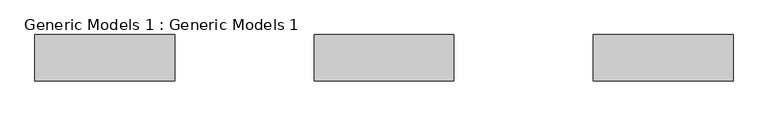
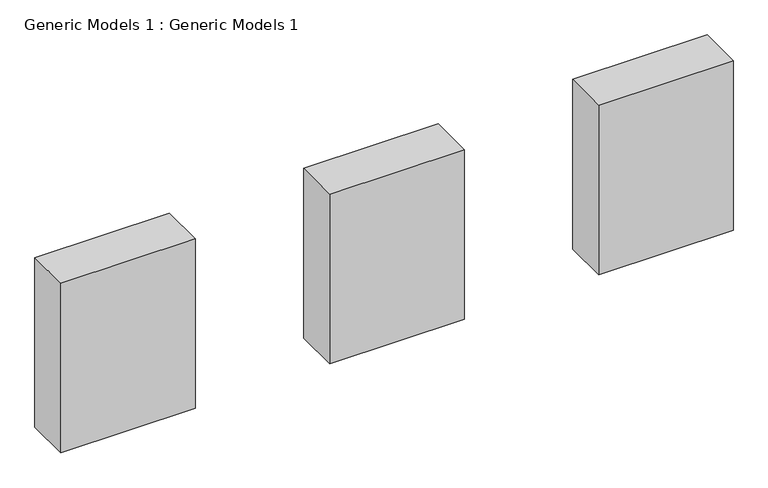
"""IFC4 building model written with IfcOpenShell, lengths in millimetres: proxy geometry, Generic Models 1 : Generic Models 1."""

from ifc_helpers import new_model, si_unit, frame, origin, place, context, project, spatial, polyline, outline, extrude, source, transform, mapped, element, save


def generic_models_1_generic_models_1_0d6a6266(model_context):
    return source(origin(), model_context, "Body", "SweptSolid", [
        extrude(outline(polyline([(-7718.7497054, -8164.8977377), (-8633.1497054, -8164.8977377), (-8633.1497054, -7860.0977377), (-7718.7497054, -7860.0977377), (-7718.7497054, -8164.8977377)])), frame((0.0, 0.0, 129.9820609), z_axis=(0.0, 0.0, 1.0), x_axis=(1.0, 0.0, 0.0)), (0.0, 0.0, 1.0), 1219.2),
        extrude(outline(polyline([(-5889.9497054, -8164.8977377), (-6804.3497054, -8164.8977377), (-6804.3497054, -7860.0977377), (-5889.9497054, -7860.0977377), (-5889.9497054, -8164.8977377)])), frame((0.0, 0.0, 129.9820609), z_axis=(0.0, 0.0, 1.0), x_axis=(1.0, 0.0, 0.0)), (0.0, 0.0, 1.0), 1219.2),
        extrude(outline(polyline([(-4061.1497054, -8164.8977377), (-4975.5497054, -8164.8977377), (-4975.5497054, -7860.0977377), (-4061.1497054, -7860.0977377), (-4061.1497054, -8164.8977377)])), frame((0.0, 0.0, 129.9820609), z_axis=(0.0, 0.0, 1.0), x_axis=(1.0, 0.0, 0.0)), (0.0, 0.0, 1.0), 1219.2),
    ])


if __name__ == "__main__":
    model = new_model("IFC4")
    model_context = context("Model", 3, world=origin())
    ifc_project = project(units=[si_unit("LENGTHUNIT", "METRE", prefix="MILLI")], contexts=[model_context])
    site = spatial("IfcSite", under=ifc_project)
    building = spatial("IfcBuilding", under=site)
    placement = place(None, origin())
    generic_models_1_generic_models_1_shape = generic_models_1_generic_models_1_0d6a6266(model_context)
    element("IfcBuildingElementProxy", 1, Name="Generic Models 1 : Generic Models 1", ObjectType="Generic Models 1 : Generic Models 1", at=placement, inside=building, context=model_context, shape_type="MappedRepresentation", body=[
        mapped(generic_models_1_generic_models_1_shape, transform((0.0, 0.0, 0.0), x_axis=(1.0, 0.0, 0.0), y_axis=(0.0, 1.0, 0.0), z_axis=(0.0, 0.0, 1.0))),
    ])
    save(model, "model.ifc")

# Revit data of these elements
# Element 1 (IfcBuildingElementProxy, "Generic Models 1 : Generic Models 1")
#   Materials on its faces: "Parking Stripe"
# Materials
#   "Parking Stripe": class "Paint", colour RGB 250 250 91, transparency 0, Cost = 0
